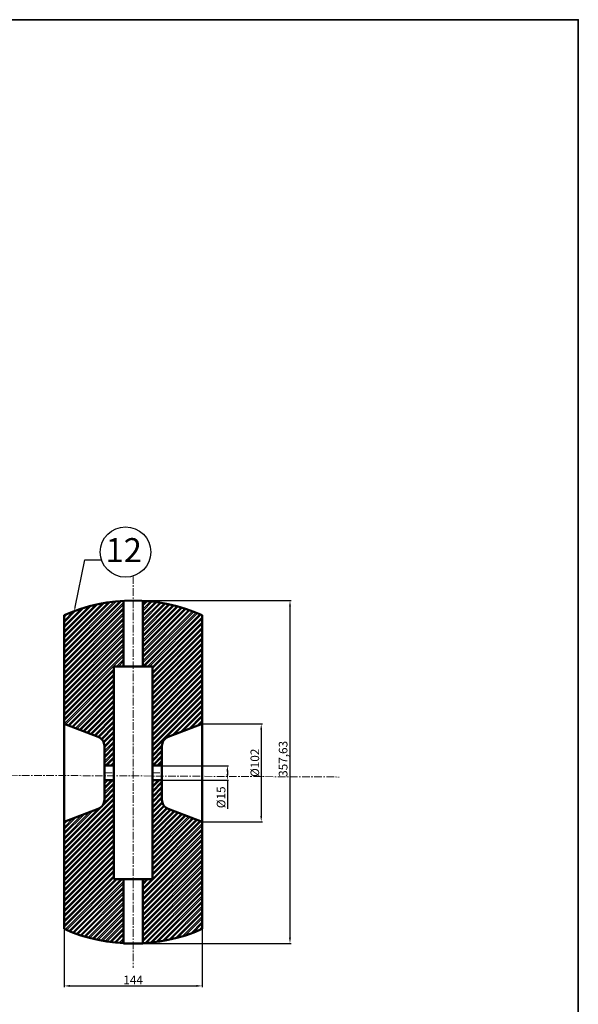
# Model space of a CAD drawing. Units: millimetres. Extents: x -282 to 2335, y -1129 to 664.
# Tile 8 of 8: x 1752 to 2335, y -363 to 664. Entities that reach past the tile are written whole.
import ezdxf
from ezdxf import colors
from ezdxf.entities.mleader import LeaderData, LeaderLine
from ezdxf.math import Vec2, Vec3

# ---------------------------------------------------------------- set-up
doc = ezdxf.new("R2010")
doc.units = ezdxf.units.MM
doc.header["$LTSCALE"] = 0.5
doc.linetypes.add('CENTER', pattern=[50.8, 31.75, -6.35, 6.35, -6.35])
for name, color, linetype, lineweight in [('M-CNTR', 1, 'CENTER', 18), ('M-DIMS', 2, 'Continuous', 25), ('M-HATC', 8, 'Continuous', 18), ('M-OUTL', 7, 'Continuous', 50), ('M-TEXT', 3, 'Continuous', 25), ('M-TTLB', 7, 'Continuous', 35)]:
    doc.layers.add(name, color=color, linetype=linetype, lineweight=lineweight)
doc.styles.get("Standard").update_dxf_attribs({"font": 'arial.ttf'})
doc.dimstyles.new('ISO-25', dxfattribs={"dimtxt": 9, "dimasz": 6, "dimexe": 1.25, "dimexo": 0.625, "dimtad": 1, "dimtxsty": 'Standard', "dimcen": 2.5, "dimadec": 0, "dimazin": 0, "dimtfac": 1, "dimtofl": 0, "dimtmove": 0, "dimatfit": 3, "dimfxl": 1, "dimarcsym": 0})

# ---------------------------------------------------------------- blocks, each defined once
blk = doc.blocks.new('*D106')
at = {"layer": 'Defpoints', "color": 0, "ltscale": 0.5, "transparency": 16777216}
for p in [(1870.8, 57.9), (1870.8, -299.8), (2034.3, -299.8)]:
    blk.add_point(p, dxfattribs=at)
at = {"layer": 'M-DIMS', "color": 0, "lineweight": -2, "ltscale": 0.5, "transparency": 16777216}
for p, q in [((1871.4, 57.9), (2035.6, 57.9)), ((2034.3, 51.9), (2034.3, -293.8)), ((1871.4, -299.8), (2035.6, -299.8))]:
    blk.add_line(p, q, dxfattribs=at)
at = {"layer": 'M-DIMS', "color": 0, "ltscale": 0.5, "transparency": 16777216}
for points in [[(2033.3, 51.9), (2035.3, 51.9), (2034.3, 57.9)], [(2033.3, -293.8), (2035.3, -293.8), (2034.3, -299.8)]]:
    blk.add_solid(points, dxfattribs=at)
at = {"layer": 'M-DIMS', "color": 0, "ltscale": 0.5, "transparency": 16777216, "insert": (2028.3, -107.2), "char_height": 9, "attachment_point": 5, "rotation": 90}
blk.add_mtext('357,63', dxfattribs=at)
blk = doc.blocks.new('*D107')
at = {"layer": 'Defpoints', "color": 0, "ltscale": 0.5, "transparency": 16777216}
for p in [(1942.8, -70.8), (1942.8, -172.8), (2004.3, -172.8)]:
    blk.add_point(p, dxfattribs=at)
at = {"layer": 'M-DIMS', "color": 0, "lineweight": -2, "ltscale": 0.5, "transparency": 16777216}
for p, q in [((1943.4, -70.8), (2005.5, -70.8)), ((2004.3, -76.8), (2004.3, -166.8)), ((1943.4, -172.8), (2005.5, -172.8))]:
    blk.add_line(p, q, dxfattribs=at)
at = {"layer": 'M-DIMS', "color": 0, "ltscale": 0.5, "transparency": 16777216}
for points in [[(2003.3, -76.8), (2005.3, -76.8), (2004.3, -70.8)], [(2003.3, -166.8), (2005.3, -166.8), (2004.3, -172.8)]]:
    blk.add_solid(points, dxfattribs=at)
at = {"layer": 'M-DIMS', "color": 0, "ltscale": 0.5, "transparency": 16777216, "insert": (1998.8, -111.3), "char_height": 9, "attachment_point": 5, "rotation": 90}
blk.add_mtext('%%C102', dxfattribs=at)
blk = doc.blocks.new('*D108')
at = {"layer": 'Defpoints', "color": 0, "ltscale": 0.5, "transparency": 16777216}
for p in [(1900.8, -114.3), (1900.8, -129.3), (1969, -129.3)]:
    blk.add_point(p, dxfattribs=at)
at = {"layer": 'M-DIMS', "color": 0, "lineweight": -2, "ltscale": 0.5, "transparency": 16777216}
for p, q in [((1901.4, -114.3), (1970.3, -114.3)), ((1969, -120.3), (1969, -123.3)), ((1901.4, -129.3), (1970.3, -129.3)), ((1969, -129.3), (1969, -159.3))]:
    blk.add_line(p, q, dxfattribs=at)
at = {"layer": 'M-DIMS', "color": 0, "ltscale": 0.5, "transparency": 16777216}
for points in [[(1968, -120.3), (1970, -120.3), (1969, -114.3)], [(1968, -123.3), (1970, -123.3), (1969, -129.3)]]:
    blk.add_solid(points, dxfattribs=at)
at = {"layer": 'M-DIMS', "color": 0, "ltscale": 0.5, "transparency": 16777216, "insert": (1963.6, -147.3), "char_height": 9, "attachment_point": 5, "rotation": 90}
blk.add_mtext('%%C15', dxfattribs=at)
blk = doc.blocks.new('*D109')
at = {"layer": 'Defpoints', "color": 0, "ltscale": 0.5, "transparency": 16777216}
for p in [(1798.8, -236.3), (1942.8, -236.3), (1942.8, -344)]:
    blk.add_point(p, dxfattribs=at)
at = {"layer": 'M-DIMS', "color": 0, "lineweight": -2, "ltscale": 0.5, "transparency": 16777216}
for p, q in [((1798.8, -236.9), (1798.8, -345.3)), ((1942.8, -236.9), (1942.8, -345.3)), ((1804.8, -344), (1936.8, -344))]:
    blk.add_line(p, q, dxfattribs=at)
at = {"layer": 'M-DIMS', "color": 0, "ltscale": 0.5, "transparency": 16777216}
for points in [[(1804.8, -343), (1804.8, -345), (1798.8, -344)], [(1936.8, -343), (1936.8, -345), (1942.8, -344)]]:
    blk.add_solid(points, dxfattribs=at)
at = {"layer": 'M-DIMS', "color": 0, "ltscale": 0.5, "transparency": 16777216, "insert": (1870.8, -338.9), "char_height": 9, "attachment_point": 5}
blk.add_mtext('144', dxfattribs=at)

msp = doc.modelspace()

# ---------------------------------------------------------------- hatches: boundary and pattern name
at = {"layer": 'M-HATC', "ltscale": 0.5}
h = msp.add_hatch(dxfattribs=at)
h.set_pattern_fill('ANSI32', color=256, scale=0.4)
h.paths.add_polyline_path([(1860.777, 57.59, 0.08985516), (1798.777, 42.734), (1798.777, -70.76), (1834.337, -84.307, -0.31120467), (1840.777, -93.652), (1840.777, -114.26), (1850.777, -114.26), (1850.777, -10.76), (1860.777, -10.76)])
h.paths.add_polyline_path([(1942.777, 42.734, 0.08985516), (1880.777, 57.59), (1880.777, -10.76), (1890.777, -10.76), (1890.777, -114.26), (1900.777, -114.26), (1900.777, -93.652, -0.31120467), (1907.217, -84.307), (1942.777, -70.76)])
h.paths.add_polyline_path([(1850.777, -129.26), (1840.777, -129.26), (1840.777, -149.869, -0.31120467), (1834.337, -159.214), (1798.777, -172.76), (1798.777, -284.624, 0.08985516), (1860.777, -299.481), (1860.777, -232.76), (1850.777, -232.76)])
h.paths.add_polyline_path([(1942.777, -172.76), (1907.217, -159.214, -0.31120467), (1900.777, -149.869), (1900.777, -129.26), (1890.777, -129.26), (1890.777, -232.76), (1880.777, -232.76), (1880.777, -299.481, 0.08985516), (1942.777, -284.624)])

# ---------------------------------------------------------------- linework, layer by layer
at = {"layer": 'M-CNTR', "ltscale": 0.5}
for p, q in [((1870.777, 83.408), (1870.777, -325.299)), ((1246.826, -121.76), (2085.572, -126.112)), ((1840.777, -121.76), (1850.777, -121.76)), ((1890.777, -121.76), (1900.777, -121.76))]:
    msp.add_line(p, q, dxfattribs=at)
at = {"layer": 'M-OUTL', "ltscale": 0.5}
for p, q in [((1860.777, 57.59), (1860.777, -10.76)), ((1880.777, 57.59), (1880.777, -10.76)), ((1798.777, 42.734), (1798.777, -284.624)), ((1942.777, -284.624), (1942.777, 42.734)), ((1850.777, -10.76), (1850.777, -232.76)), ((1850.777, -10.76), (1890.777, -10.76)), ((1890.777, -10.76), (1890.777, -232.76)), ((1834.337, -84.307), (1798.777, -70.76)), ((1942.777, -70.76), (1907.217, -84.307)), ((1840.777, -93.652), (1840.777, -149.869)), ((1900.777, -93.652), (1900.777, -149.869)), ((1840.777, -114.26), (1850.777, -114.26)), ((1890.777, -114.26), (1900.777, -114.26)), ((1840.777, -129.26), (1850.777, -129.26)), ((1890.777, -129.26), (1900.777, -129.26)), ((1798.777, -172.76), (1834.337, -159.214)), ((1942.777, -172.76), (1907.217, -159.214)), ((1850.777, -232.76), (1890.777, -232.76)), ((1860.777, -299.76), (1860.777, -232.76)), ((1880.777, -299.76), (1880.777, -232.76)), ((1860.777, -299.76), (1880.777, -299.76))]:
    msp.add_line(p, q, dxfattribs=at)
for centre, radius, start, end in [((1870.777, -120.945), 178.815, 66.256004, 113.743996), ((1830.777, -93.652), 10, 0, 69.145542), ((1910.777, -93.652), 10, 110.854458, 180), ((1830.777, -149.869), 10, 290.854458, 0), ((1910.777, -149.869), 10, 180, 249.145542), ((1870.777, -120.945), 178.815, 246.256004, 293.743996)]:
    msp.add_arc(centre, radius, start, end, dxfattribs=at)
at = {"layer": 'M-TEXT'}
msp.add_circle((1862.795, 108.511), 26.287, dxfattribs=at)
at = {"layer": 'M-TTLB', "ltscale": 0.5}
msp.add_lwpolyline([(-281.776, 663.767), (2334.915, 663.767), (2334.915, -1128.523), (-281.776, -1128.523)], close=True, dxfattribs=at)

# ---------------------------------------------------------------- texts
at = {"layer": 'M-TEXT', "insert": (1848.462, 123.051), "char_height": 25, "attachment_point": 1}
msp.add_mtext_dynamic_manual_height_columns('\\pxqc;12', width=25, gutter_width=12.5, heights=[7.196], dxfattribs=at)

# ---------------------------------------------------------------- dimensions: what is measured, and where the dimension line sits
at = {"layer": 'M-DIMS', "ltscale": 0.5}
dim = msp.add_linear_dim(base=(2034.31, -299.76), p1=(1870.777, 57.87), p2=(1870.777, -299.76), angle=90, dimstyle='ISO-25', override={"dimclrd": 0, "dimclre": 0, "dimclrt": 0}, dxfattribs=at)
dim.commit()
dim.dimension.update_dxf_attribs({"geometry": '*D106', "text_midpoint": (2034.31, -107.22), "dimtype": 160})
for base, p1, p2, picture, middle in [((2004.274, -172.76), (1942.777, -70.76), (1942.777, -172.76), '*D107', (2004.274, -111.319)), ((1969.049, -129.26), (1900.777, -114.26), (1900.777, -129.26), '*D108', (1969.049, -147.261))]:
    dim = msp.add_linear_dim(base=base, p1=p1, p2=p2, angle=90, text='%%C<>', dimstyle='ISO-25', override={"dimclrd": 0, "dimclre": 0, "dimclrt": 0}, dxfattribs=at)
    dim.commit()
    dim.dimension.update_dxf_attribs({"geometry": picture, "text_midpoint": middle, "dimtype": 160})
dim = msp.add_linear_dim(base=(1942.777, -344.008), p1=(1798.777, -236.301), p2=(1942.777, -236.301), dimstyle='ISO-25', override={"dimclrd": 0, "dimclre": 0, "dimclrt": 0}, dxfattribs=at)
dim.commit()
dim.dimension.update_dxf_attribs({"geometry": '*D109', "text_midpoint": (1870.777, -344.008), "dimtype": 160})

# ---------------------------------------------------------------- leaders
at = {"layer": 'M-TEXT', "ltscale": 0.5}
ml = msp.add_multileader_mtext('Standard', dxfattribs=at)
ml.set_content('', color=256)
ml.set_leader_properties()
ml.build(insert=Vec2(0, 0))
ctx = ml.context
ctx.base_point, ctx.plane_origin = Vec3(1837.676, 100.404), Vec3(1813.633, 57.59)
notes = []
notes.append((ctx, [(0, (1, 1, 0), (1820.401, 100.404), (1, 0), 17.275, [(0, [(1809.463, 47.029)], 0, [])])]))
ctx.mtext.insert, ctx.mtext.flow_direction = Vec3(1839.676, 102.404), 5
for ctx, leaders in notes:
    for number, flags, end, landing, length, lines in leaders:
        leader = LeaderData()
        leader.index, (leader.has_last_leader_line, leader.has_dogleg_vector, leader.attachment_direction) = number, flags
        leader.last_leader_point, leader.dogleg_vector, leader.dogleg_length = Vec3(end), Vec3(landing), length
        for number, points, colour, breaks in lines:
            line = LeaderLine()
            line.index, line.vertices, line.color, line.breaks = number, Vec3.list(points), colors.encode_raw_color(colour), breaks
            leader.lines.append(line)
        ctx.leaders.append(leader)

doc.saveas('drawing.dxf')
